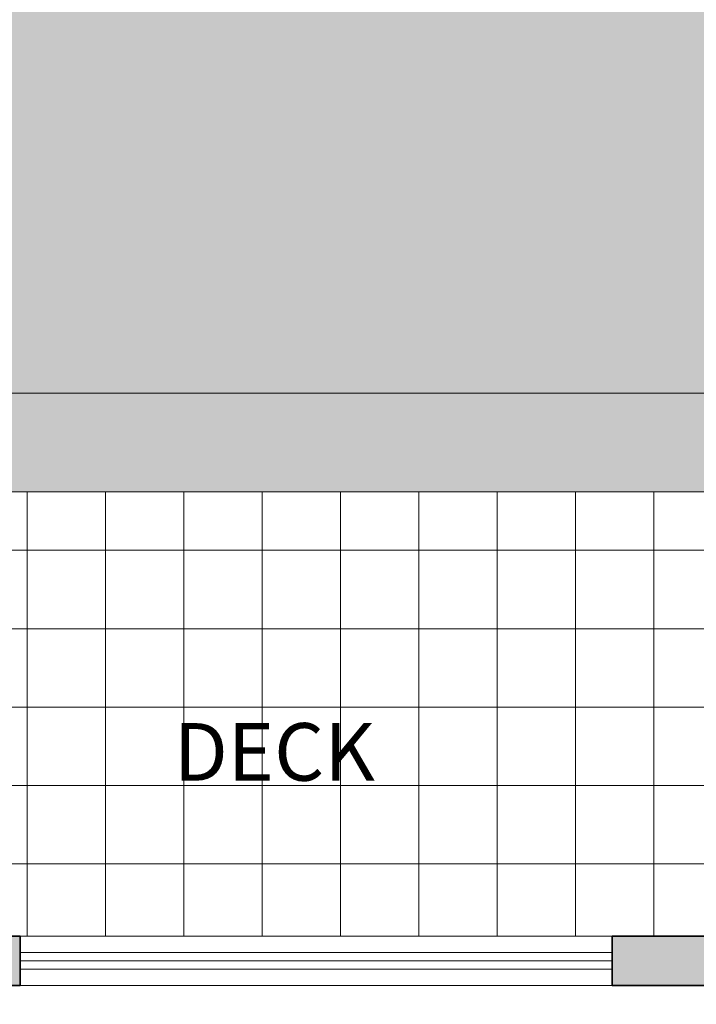
# Model space of a CAD drawing. Units: inches. Extents: x 84 to 1044, y -280 to 906.
# Tile 79 of 105: x 733 to 815, y 326 to 445. Entities that reach past the tile are written whole.
import ezdxf

# ---------------------------------------------------------------- set-up
doc = ezdxf.new("R2010")
doc.units = ezdxf.units.IN
for name, color, linetype, lineweight in [('A-ANNO-DIMS', 2, 'Continuous', 18), ('A-AREA-IDEN', 7, 'Continuous', 13), ('A-STAIRCASE', 144, 'Continuous', 18), ('WALL', 250, 'Continuous', 35), ('WINDOW', 160, 'Continuous', 13)]:
    doc.layers.add(name, color=color, linetype=linetype, lineweight=lineweight)
for name, color, linetype, lineweight, true_color in [('A-FLOR-PATT', 251, 'Continuous', 9, 0x705861), ('A-FLOR-STRS-PATT', 35, 'Continuous', 9, 0x947764), ('A-WALL-PATT', 251, 'Continuous', 9, 0x636466), ('L-PLNT-PATT', 9, 'Continuous', 9, 0xafd9aa)]:
    doc.layers.add(name, color=color, linetype=linetype, lineweight=lineweight, true_color=true_color)
doc.styles.add('1-100DIM', font='txt', dxfattribs={"height": 0.3})
doc.styles.get("Standard").update_dxf_attribs({"font": 'arial.ttf'})
doc.dimstyles.get("Standard").update_dxf_attribs({"dimtxt": 0.18, "dimasz": 0.18, "dimexe": 0.18, "dimexo": 0.0625, "dimgap": 0.09, "dimtad": 0, "dimtih": 1, "dimtoh": 1, "dimdec": 4, "dimzin": 0, "dimdsep": 46, "dimtxsty": 'Standard', "dimcen": 0.09, "dimadec": 0, "dimazin": 0, "dimtfac": 1, "dimtdec": 4, "dimtofl": 0, "dimtmove": 0, "dimatfit": 3, "dimfxl": 1, "dimtolj": 1, "dimtzin": 0, "dimarcsym": 0})

# ---------------------------------------------------------------- blocks, each defined once
blk = doc.blocks.new('*D62')
at = {"layer": 'A-ANNO-DIMS', "color": 0, "lineweight": -2, "transparency": 16777216}
for p, q in [((203.18, 709.18), (203.18, 905.9)), ((203.36, 905.72), (549.23, 905.72)), ((895.89, 905.72), (550.02, 905.72)), ((896.07, 400.18), (896.07, 905.9))]:
    blk.add_line(p, q, dxfattribs=at)
at = {"layer": 'A-ANNO-DIMS', "color": 0, "transparency": 16777216}
for points in [[(203.36, 905.75), (203.36, 905.69), (203.18, 905.72)], [(895.89, 905.75), (895.89, 905.69), (896.07, 905.72)]]:
    blk.add_solid(points, dxfattribs=at)
at = {"layer": 'Defpoints', "color": 0, "transparency": 16777216}
for p in [(896.07, 905.72), (203.18, 709.12), (896.07, 400.12)]:
    blk.add_point(p, dxfattribs=at)
at = {"layer": 'A-ANNO-DIMS', "color": 0, "transparency": 16777216, "insert": (549.63, 905.72), "char_height": 0.18, "attachment_point": 5}
blk.add_mtext('\\A1;692.9', dxfattribs=at)

msp = doc.modelspace()

# ---------------------------------------------------------------- hatches: boundary and pattern name
at = {"layer": 'A-FLOR-PATT', "transparency": 33554597}
h = msp.add_hatch(dxfattribs=at)
h.set_pattern_fill('ANSI37', color=256, scale=3, angle=45)
h.paths.add_polyline_path([(833.074, 388.12), (704.074, 388.12), (704.074, 370.12), (695.074, 370.12), (695.074, 334.12), (732.574, 334.12), (804.574, 334.12), (833.074, 334.12), (833.074, 364.12)])
at = {"layer": 'A-FLOR-STRS-PATT', "transparency": 33554567}
h = msp.add_hatch(color=256, dxfattribs=at)
h.dxf.hatch_style = 1
h.paths.add_polyline_path([(833.074, 400.12), (704.074, 400.12), (704.074, 388.12), (833.074, 388.12)])
at = {"layer": 'A-WALL-PATT', "transparency": 33554597}
h = msp.add_hatch(color=256, dxfattribs=at)
h.dxf.hatch_style = 1
h.paths.add_polyline_path([(671.074, 100.12), (647.074, 100.12), (647.074, 160.12), (641.074, 160.12), (620.824, 160.12), (620.824, 151.12), (638.074, 151.12), (638.074, 91.12), (671.074, 91.12)])
h.paths.add_polyline_path([(791.074, 100.12), (743.074, 100.12), (743.074, 91.12), (791.074, 91.12)])
h.paths.add_polyline_path([(896.074, 346.12), (887.074, 346.12), (887.074, 334.12), (870.955, 334.12), (833.074, 334.12), (804.574, 334.12), (804.574, 328.12), (887.074, 328.12), (887.074, 100.12), (863.074, 100.12), (863.074, 91.12), (896.074, 91.12)])
h.paths.add_polyline_path([(507.574, 154.729), (507.574, 160.12), (464.074, 160.12), (464.074, 247.12), (641.074, 247.12), (641.074, 208.12), (647.074, 208.12), (647.074, 328.12), (659.074, 328.12), (659.074, 334.12), (617.074, 334.12), (617.074, 328.12), (641.074, 328.12), (641.074, 256.12), (545.074, 256.12), (545.074, 328.12), (569.074, 328.12), (569.074, 334.12), (518.074, 334.12), (518.074, 325.12), (536.074, 325.12), (536.074, 256.12), (464.074, 256.12), (464.074, 325.12), (482.074, 325.12), (482.074, 334.12), (455.074, 334.12), (455.074, 160.12), (413.127, 160.12), (413.127, 151.12), (455.074, 151.12), (455.074, 91.12), (464.074, 91.12), (464.074, 151.12), (507.574, 151.12)])
h.paths.add_polyline_path([(572.824, 160.12), (555.574, 160.12), (555.574, 151.12), (572.824, 151.12)], flags=17)
h.paths.add_polyline_path([(341.127, 160.12), (299.179, 160.12), (299.179, 211.12), (294.179, 211.12), (290.179, 211.12), (290.179, 151.12), (341.127, 151.12)])
h.paths.add_polyline_path([(299.179, 256.12), (212.179, 256.12), (212.179, 274.12), (203.179, 274.12), (203.179, 247.12), (299.179, 247.12)])
h.paths.add_polyline_path([(212.179, 514.12), (398.074, 514.12), (398.074, 519.12), (398.074, 520.12), (212.179, 520.12), (212.179, 574.12), (203.179, 574.12), (203.179, 310.12), (212.179, 310.12), (212.179, 328.12), (290.179, 328.12), (290.179, 292.12), (299.179, 292.12), (299.179, 328.12), (332.179, 328.12), (332.179, 334.12), (212.179, 334.12)])
h.paths.add_polyline_path([(287.127, 709.12), (203.179, 709.12), (203.179, 646.12), (212.179, 646.12), (212.179, 700.12), (287.127, 700.12)])
h.paths.add_polyline_path([(470.074, 709.12), (359.127, 709.12), (359.127, 700.12), (434.074, 700.12), (434.074, 574.12), (440.074, 574.12), (440.074, 622.12), (464.074, 622.12), (464.074, 628.12), (440.074, 628.12), (440.074, 700.12), (470.074, 700.12)])
h.paths.add_polyline_path([(572.074, 709.12), (506.074, 709.12), (506.074, 700.12), (536.074, 700.12), (536.074, 628.12), (494.074, 628.12), (494.074, 622.12), (536.074, 622.12), (536.074, 520.12), (440.074, 520.12), (440.074, 544.12), (434.074, 544.12), (434.074, 514.12), (644.074, 514.12), (644.074, 519.12), (644.074, 544.12), (638.074, 544.12), (638.074, 520.12), (542.074, 520.12), (542.074, 622.12), (584.074, 622.12), (584.074, 628.12), (542.074, 628.12), (542.074, 700.12), (572.074, 700.12)])
h.paths.add_polyline_path([(698.074, 709.12), (608.074, 709.12), (608.074, 700.12), (638.074, 700.12), (638.074, 628.12), (614.074, 628.12), (614.074, 622.12), (638.074, 622.12), (638.074, 574.12), (644.074, 574.12), (644.074, 700.12), (698.074, 700.12)])
h.paths.add_polyline_path([(833.074, 709.12), (770.074, 709.12), (770.074, 700.12), (824.074, 700.12), (824.074, 646.12), (833.074, 646.12)])
h.paths.add_polyline_path([(833.074, 574.12), (824.074, 574.12), (824.074, 520.12), (791.244, 520.12), (712.904, 520.12), (680.074, 520.12), (680.074, 514.12), (695.074, 514.12), (695.074, 491.62), (704.074, 491.62), (704.074, 511.12), (833.074, 511.12)])
h.paths.add_polyline_path([(704.074, 419.62), (695.074, 419.62), (695.074, 370.12), (704.074, 370.12)])
h.paths.add_polyline_path([(896.074, 400.12), (833.074, 400.12), (833.074, 364.12), (839.074, 364.12), (839.074, 394.12), (887.074, 394.12), (887.074, 382.12), (896.074, 382.12)])
h.paths.add_polyline_path([(732.574, 334.12), (695.074, 334.12), (695.074, 328.12), (732.574, 328.12)])
at = {"layer": 'L-PLNT-PATT', "transparency": 33554597}
h = msp.add_hatch(color=256, dxfattribs=at)
h.dxf.hatch_style = 1
h.paths.add_polyline_path([(896.074, 511.12), (704.074, 511.12), (704.074, 491.62), (704.074, 419.62), (704.074, 400.12), (833.074, 400.12), (896.074, 400.12)])

# ---------------------------------------------------------------- linework, layer by layer
at = {"layer": 'A-STAIRCASE'}
for p, q in [((833.074, 400.12), (704.074, 400.12)), ((833.074, 388.12), (704.074, 388.12))]:
    msp.add_line(p, q, dxfattribs=at)
at = {"layer": 'WALL'}
for p, q in [((732.574, 334.12), (695.074, 334.12)), ((732.574, 334.12), (732.574, 328.12)), ((833.074, 334.12), (804.574, 334.12)), ((804.574, 334.12), (804.574, 328.12)), ((732.574, 328.12), (695.074, 328.12)), ((887.074, 328.12), (804.574, 328.12))]:
    msp.add_line(p, q, dxfattribs=at)
at = {"layer": 'WINDOW'}
for p, q in [((804.574, 334.12), (732.574, 334.12)), ((804.574, 332.12), (732.574, 332.12)), ((804.574, 331.12), (732.574, 331.12)), ((804.574, 330.12), (732.574, 330.12)), ((732.574, 328.12), (804.574, 328.12))]:
    msp.add_line(p, q, dxfattribs=at)

# ---------------------------------------------------------------- texts
at = {"layer": 'A-AREA-IDEN', "insert": (742.706, 360.012), "char_height": 7, "attachment_point": 1, "style": '1-100DIM'}
msp.add_mtext_dynamic_manual_height_columns('{\\f@Malgun Gothic|b0|i0|c0|p34;    DECK }', width=51.07953, gutter_width=15.851, heights=[0], dxfattribs=at)

# ---------------------------------------------------------------- dimensions: what is measured, and where the dimension line sits
at = {"layer": 'A-ANNO-DIMS'}
dim = msp.add_linear_dim(base=(896.074, 905.72), p1=(203.179, 709.12), p2=(896.074, 400.12), dimstyle='Standard', override={"dimdec": 1, "dimlfac": 1, "dimrnd": 0, "dimzin": 0, "dimdsep": 46, "dimlunit": 2}, dxfattribs=at)
dim.commit()
dim.dimension.update_dxf_attribs({"geometry": '*D62', "text_midpoint": (549.627, 905.72)})

doc.saveas('drawing.dxf')
